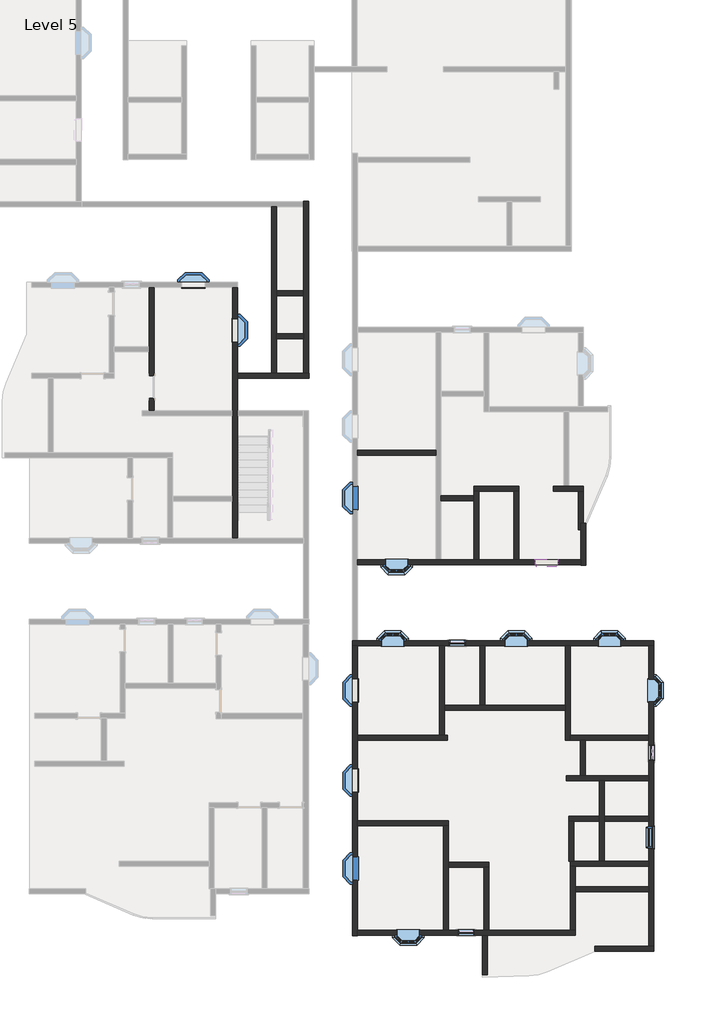
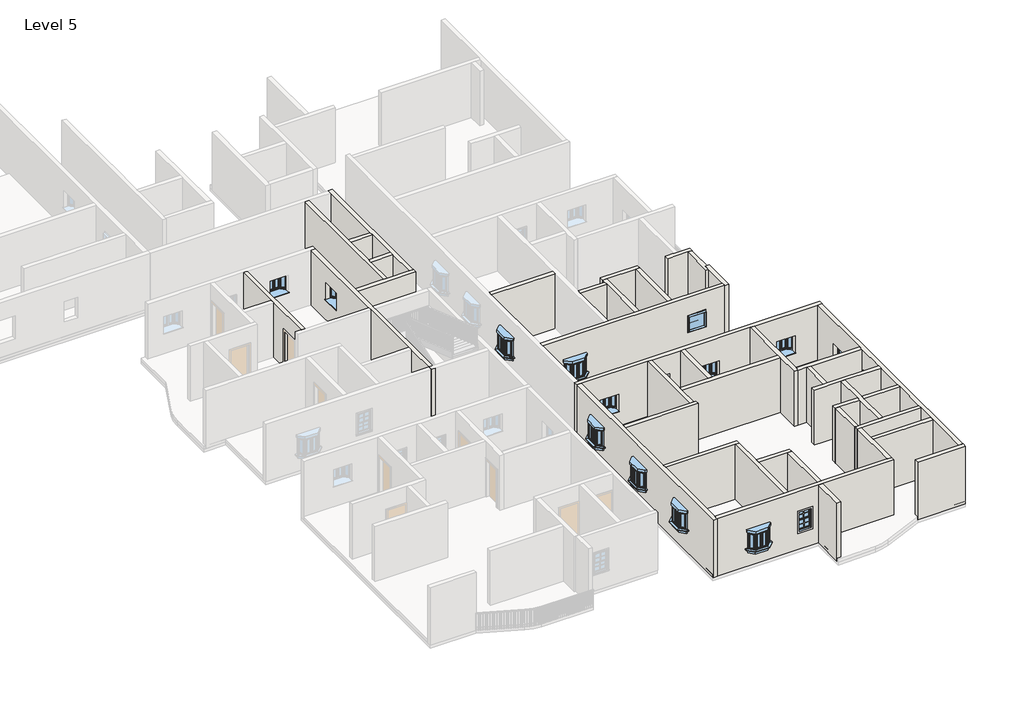
# One storey, part 2 of 14: 40 walls, 17 windows.
"""IFC4 building model written with IfcOpenShell, lengths in millimetres."""

from ifc_helpers import new_model, si_unit, frame, origin, place, context, project, spatial, polyline, outline, extrude, faceted_brep, transform, mapped, element, save
from components import window_910x910mm_67ef725a, window_8debb0fa, windows_sgl_w_glazing_bars_910x910mm_256712d0

model = new_model("IFC4")

# Units and contexts
model_context = context("Model", 3, world=origin())
ifc_project = project(units=[si_unit("LENGTHUNIT", "METRE", prefix="MILLI")], contexts=[model_context])

# Site, building, storey
site = spatial("IfcSite", under=ifc_project)
building = spatial("IfcBuilding", under=site)
storey = spatial("IfcBuildingStorey", under=building, Name="Level 5", Elevation=12192.0)

# Walls
placement = place(None, origin())
element("IfcWall", 1, ObjectType="4.5\" p", at=placement, inside=storey, context=model_context, shape_type="SweptSolid", body=[
    extrude(outline(polyline([(6070.4380523, -28382.7374148), (6070.4380523, -26796.6042694), (6273.6380523, -26796.6042694), (6273.6380523, -28382.7374148), (6070.4380523, -28382.7374148)])), frame((0.0, 0.0, 12192.0), z_axis=(0.0, 0.0, 1.0), x_axis=(1.0, 0.0, 0.0)), (0.0, 0.0, 1.0), 3048.0),
])
element("IfcWall", 2, ObjectType="4.5\" p", at=placement, inside=storey, context=model_context, shape_type="Brep", body=[
    faceted_brep([(10639.6896214, -27431.6042694, 12192.0), (13030.0380523, -27431.6042694, 12192.0), (13030.0380523, -27431.6042694, 15240.0), (10639.6896214, -27431.6042694, 15240.0), (10639.6896214, -27228.4042694, 12192.0), (10639.6896214, -27228.4042694, 15240.0), (12814.1380523, -27228.4042694, 15240.0), (13017.3380523, -27228.4042694, 15240.0), (13030.0380523, -27228.4042694, 15240.0), (13030.0380523, -27228.4042694, 12192.0), (13017.3380523, -27228.4042694, 12192.0), (12814.1380523, -27228.4042694, 12192.0)], [[[0, 1, 2, 3]], [[4, 5, 6, 7, 8, 9, 10, 11]], [[1, 0, 4, 11, 10, 9]], [[2, 1, 9, 8]], [[3, 2, 8, 7, 6, 5]], [[0, 3, 5, 4]]]),
])
element("IfcWall", 3, ObjectType="4.5\" p", at=placement, inside=storey, context=model_context, shape_type="Brep", body=[
    faceted_brep([(1015.8380523, -18878.1542694, 12192.0), (4648.0380523, -18878.1542694, 12192.0), (4648.0380523, -18878.1542694, 15240.0), (1015.8380523, -18878.1542694, 15240.0), (1015.8380523, -18674.9542694, 12192.0), (1015.8380523, -18674.9542694, 15240.0), (4336.8880523, -18674.9542694, 15240.0), (4540.0880523, -18674.9542694, 15240.0), (4648.0380523, -18674.9542694, 15240.0), (4648.0380523, -18674.9542694, 12192.0), (4540.0880523, -18674.9542694, 12192.0), (4336.8880523, -18674.9542694, 12192.0)], [[[0, 1, 2, 3]], [[4, 5, 6, 7, 8, 9, 10, 11]], [[1, 0, 4, 11, 10, 9]], [[2, 1, 9, 8]], [[3, 2, 8, 7, 6, 5]], [[0, 3, 5, 4]]]),
])
element("IfcWall", 4, ObjectType="4.5\" p", at=placement, inside=storey, context=model_context, shape_type="Brep", body=[
    faceted_brep([(4336.8880523, -15049.1042694, 12192.0), (4336.8880523, -18674.9542694, 12192.0), (4336.8880523, -18674.9542694, 15240.0), (4336.8880523, -15049.1042694, 15240.0), (4540.0880523, -15049.1042694, 12192.0), (4540.0880523, -15049.1042694, 15240.0), (4540.0880523, -17455.7542694, 15240.0), (4540.0880523, -17658.9542694, 15240.0), (4540.0880523, -18674.9542694, 15240.0), (4540.0880523, -18674.9542694, 12192.0), (4540.0880523, -17658.9542694, 12192.0), (4540.0880523, -17455.7542694, 12192.0)], [[[0, 1, 2, 3]], [[4, 5, 6, 7, 8, 9, 10, 11]], [[1, 0, 4, 11, 10, 9]], [[3, 2, 8, 7, 6, 5]], [[0, 3, 5, 4]], [[2, 1, 9, 8]]]),
])
element("IfcWall", 5, ObjectType="4.5\" p", at=placement, inside=storey, context=model_context, shape_type="Brep", body=[
    faceted_brep([(4540.0880523, -17658.9542694, 12192.0), (9442.2880523, -17658.9542694, 12192.0), (9442.2880523, -17658.9542694, 15240.0), (4540.0880523, -17658.9542694, 15240.0), (4540.0880523, -17455.7542694, 12192.0), (4540.0880523, -17455.7542694, 15240.0), (5975.1880523, -17455.7542694, 15240.0), (6178.3880523, -17455.7542694, 15240.0), (9442.2880523, -17455.7542694, 15240.0), (9442.2880523, -17455.7542694, 12192.0), (6178.3880523, -17455.7542694, 12192.0), (5975.1880523, -17455.7542694, 12192.0)], [[[0, 1, 2, 3]], [[4, 5, 6, 7, 8, 9, 10, 11]], [[1, 0, 4, 11, 10, 9]], [[3, 2, 8, 7, 6, 5]], [[0, 3, 5, 4]], [[2, 1, 9, 8]]]),
])
element("IfcWall", 6, ObjectType="4.5\" p", at=placement, inside=storey, context=model_context, shape_type="SweptSolid", body=[
    extrude(outline(polyline([(5975.1880523, -17455.7542694), (5975.1880523, -15049.1042694), (6178.3880523, -15049.1042694), (6178.3880523, -17455.7542694), (5975.1880523, -17455.7542694)])), frame((0.0, 0.0, 12192.0), z_axis=(0.0, 0.0, 1.0), x_axis=(1.0, 0.0, 0.0)), (0.0, 0.0, 1.0), 3048.0),
])
element("IfcWall", 7, ObjectType="4.5\" p", at=placement, inside=storey, context=model_context, shape_type="Brep", body=[
    faceted_brep([(9442.2880523, -15049.1042694, 12192.0), (9442.2880523, -17455.7542694, 12192.0), (9442.2880523, -17658.9542694, 12192.0), (9442.2880523, -18871.8042694, 12192.0), (9442.2880523, -18871.8042694, 15240.0), (9442.2880523, -17658.9542694, 15240.0), (9442.2880523, -17455.7542694, 15240.0), (9442.2880523, -15049.1042694, 15240.0), (9645.4880523, -15049.1042694, 12192.0), (9645.4880523, -15049.1042694, 15240.0), (9645.4880523, -18668.6042694, 15240.0), (9645.4880523, -18871.8042694, 15240.0), (9645.4880523, -18871.8042694, 12192.0), (9645.4880523, -18668.6042694, 12192.0)], [[[0, 1, 2, 3, 4, 5, 6, 7]], [[8, 9, 10, 11, 12, 13]], [[3, 2, 1, 0, 8, 13, 12]], [[7, 6, 5, 4, 11, 10, 9]], [[0, 7, 9, 8]], [[4, 3, 12, 11]]]),
])
element("IfcWall", 8, ObjectType="4.5\" p", at=placement, inside=storey, context=model_context, shape_type="Brep", body=[
    faceted_brep([(1015.8380523, -22345.2542694, 12192.0), (4489.2880523, -22345.2542694, 12192.0), (4692.4880523, -22345.2542694, 12192.0), (4692.4880523, -22345.2542694, 15240.0), (4489.2880523, -22345.2542694, 15240.0), (1015.8380523, -22345.2542694, 15240.0), (1015.8380523, -22142.0542694, 12192.0), (1015.8380523, -22142.0542694, 15240.0), (4692.4880523, -22142.0542694, 15240.0), (4692.4880523, -22142.0542694, 12192.0)], [[[0, 1, 2, 3, 4, 5]], [[6, 7, 8, 9]], [[2, 1, 0, 6, 9]], [[5, 4, 3, 8, 7]], [[0, 5, 7, 6]], [[3, 2, 9, 8]]]),
])
element("IfcWall", 9, ObjectType="4.5\" p", at=placement, inside=storey, context=model_context, shape_type="Brep", body=[
    faceted_brep([(4489.2880523, -22345.2542694, 12192.0), (4489.2880523, -26580.7042694, 12192.0), (4489.2880523, -26580.7042694, 15240.0), (4489.2880523, -22345.2542694, 15240.0), (4692.4880523, -22345.2542694, 12192.0), (4692.4880523, -22345.2542694, 15240.0), (4692.4880523, -23818.4542694, 15240.0), (4692.4880523, -24021.6542694, 15240.0), (4692.4880523, -26580.7042694, 15240.0), (4692.4880523, -26580.7042694, 12192.0), (4692.4880523, -24021.6542694, 12192.0), (4692.4880523, -23818.4542694, 12192.0)], [[[0, 1, 2, 3]], [[4, 5, 6, 7, 8, 9, 10, 11]], [[1, 0, 4, 11, 10, 9]], [[3, 2, 8, 7, 6, 5]], [[0, 3, 5, 4]], [[2, 1, 9, 8]]]),
])
element("IfcWall", 10, ObjectType="4.5\" p", at=placement, inside=storey, context=model_context, shape_type="Brep", body=[
    faceted_brep([(4692.4880523, -24021.6542694, 12192.0), (6127.5880523, -24021.6542694, 12192.0), (6330.7880523, -24021.6542694, 12192.0), (6330.7880523, -24021.6542694, 15240.0), (6127.5880523, -24021.6542694, 15240.0), (4692.4880523, -24021.6542694, 15240.0), (4692.4880523, -23818.4542694, 12192.0), (4692.4880523, -23818.4542694, 15240.0), (6330.7880523, -23818.4542694, 15240.0), (6330.7880523, -23818.4542694, 12192.0)], [[[0, 1, 2, 3, 4, 5]], [[6, 7, 8, 9]], [[2, 1, 0, 6, 9]], [[5, 4, 3, 8, 7]], [[0, 5, 7, 6]], [[3, 2, 9, 8]]]),
])
element("IfcWall", 11, ObjectType="4.5\" p", at=placement, inside=storey, context=model_context, shape_type="SweptSolid", body=[
    extrude(outline(polyline([(6127.5880523, -26580.7042694), (6127.5880523, -24021.6542694), (6330.7880523, -24021.6542694), (6330.7880523, -26580.7042694), (6127.5880523, -26580.7042694)])), frame((0.0, 0.0, 12192.0), z_axis=(0.0, 0.0, 1.0), x_axis=(1.0, 0.0, 0.0)), (0.0, 0.0, 1.0), 3048.0),
])
element("IfcWall", 12, ObjectType="4.5\" p", at=placement, inside=storey, context=model_context, shape_type="Brep", body=[
    faceted_brep([(9645.4880523, -18871.8042694, 12192.0), (10051.8880523, -18871.8042694, 12192.0), (10255.0880523, -18871.8042694, 12192.0), (12814.1380523, -18871.8042694, 12192.0), (12814.1380523, -18871.8042694, 15240.0), (10255.0880523, -18871.8042694, 15240.0), (10051.8880523, -18871.8042694, 15240.0), (9645.4880523, -18871.8042694, 15240.0), (9645.4880523, -18668.6042694, 12192.0), (9645.4880523, -18668.6042694, 15240.0), (12814.1380523, -18668.6042694, 15240.0), (12814.1380523, -18668.6042694, 12192.0)], [[[0, 1, 2, 3, 4, 5, 6, 7]], [[8, 9, 10, 11]], [[3, 2, 1, 0, 8, 11]], [[7, 6, 5, 4, 10, 9]], [[0, 7, 9, 8]], [[4, 3, 11, 10]]]),
])
element("IfcWall", 13, ObjectType="4.5\" p", at=placement, inside=storey, context=model_context, shape_type="SweptSolid", body=[
    extrude(outline(polyline([(10051.8880523, -20313.2542694), (10051.8880523, -18871.8042694), (10255.0880523, -18871.8042694), (10255.0880523, -20313.2542694), (10051.8880523, -20313.2542694)])), frame((0.0, 0.0, 12192.0), z_axis=(0.0, 0.0, 1.0), x_axis=(1.0, 0.0, 0.0)), (0.0, 0.0, 1.0), 3048.0),
])
element("IfcWall", 14, ObjectType="4.5\" p", at=placement, inside=storey, context=model_context, shape_type="Brep", body=[
    faceted_brep([(12814.1380523, -20313.2542694, 12192.0), (10255.0880523, -20313.2542694, 12192.0), (10051.8880523, -20313.2542694, 12192.0), (9486.7380523, -20313.2542694, 12192.0), (9486.7380523, -20313.2542694, 15240.0), (10051.8880523, -20313.2542694, 15240.0), (10255.0880523, -20313.2542694, 15240.0), (12814.1380523, -20313.2542694, 15240.0), (12814.1380523, -20516.4542694, 12192.0), (12814.1380523, -20516.4542694, 15240.0), (11017.0880523, -20516.4542694, 15240.0), (10813.8880523, -20516.4542694, 15240.0), (9486.7380523, -20516.4542694, 15240.0), (9486.7380523, -20516.4542694, 12192.0), (10813.8880523, -20516.4542694, 12192.0), (11017.0880523, -20516.4542694, 12192.0)], [[[0, 1, 2, 3, 4, 5, 6, 7]], [[8, 9, 10, 11, 12, 13, 14, 15]], [[3, 2, 1, 0, 8, 15, 14, 13]], [[4, 3, 13, 12]], [[7, 6, 5, 4, 12, 11, 10, 9]], [[0, 7, 9, 8]]]),
])
element("IfcWall", 15, ObjectType="4.5\" p", at=placement, inside=storey, context=model_context, shape_type="Brep", body=[
    faceted_brep([(10813.8880523, -20516.4542694, 12192.0), (10813.8880523, -21951.5542694, 12192.0), (10813.8880523, -22154.7542694, 12192.0), (10813.8880523, -23779.5416506, 12192.0), (10813.8880523, -23779.5416506, 15240.0), (10813.8880523, -22154.7542694, 15240.0), (10813.8880523, -21951.5542694, 15240.0), (10813.8880523, -20516.4542694, 15240.0), (11017.0880523, -20516.4542694, 12192.0), (11017.0880523, -20516.4542694, 15240.0), (11017.0880523, -21951.5542694, 15240.0), (11017.0880523, -22154.7542694, 15240.0), (11017.0880523, -23779.5416506, 15240.0), (11017.0880523, -23779.5416506, 12192.0), (11017.0880523, -22154.7542694, 12192.0), (11017.0880523, -21951.5542694, 12192.0)], [[[0, 1, 2, 3, 4, 5, 6, 7]], [[8, 9, 10, 11, 12, 13, 14, 15]], [[3, 2, 1, 0, 8, 15, 14, 13]], [[7, 6, 5, 4, 12, 11, 10, 9]], [[0, 7, 9, 8]], [[4, 3, 13, 12]]]),
])
element("IfcWall", 16, ObjectType="4.5\" p", at=placement, inside=storey, context=model_context, shape_type="Brep", body=[
    faceted_brep([(12814.1380523, -23779.5416506, 12192.0), (11017.0880523, -23779.5416506, 12192.0), (10813.8880523, -23779.5416506, 12192.0), (9791.5380523, -23779.5416506, 12192.0), (9632.7880523, -23779.5416506, 12192.0), (9632.7880523, -23779.5416506, 15240.0), (9791.5380523, -23779.5416506, 15240.0), (10813.8880523, -23779.5416506, 15240.0), (11017.0880523, -23779.5416506, 15240.0), (12814.1380523, -23779.5416506, 15240.0), (12814.1380523, -23982.7416506, 12192.0), (12814.1380523, -23982.7416506, 15240.0), (9835.9880523, -23982.7416506, 15240.0), (9632.7880523, -23982.7416506, 15240.0), (9632.7880523, -23982.7416506, 12192.0), (9835.9880523, -23982.7416506, 12192.0)], [[[0, 1, 2, 3, 4, 5, 6, 7, 8, 9]], [[10, 11, 12, 13, 14, 15]], [[4, 3, 2, 1, 0, 10, 15, 14]], [[9, 8, 7, 6, 5, 13, 12, 11]], [[0, 9, 11, 10]], [[5, 4, 14, 13]]]),
])
element("IfcWall", 17, ObjectType="4.5\" p", at=placement, inside=storey, context=model_context, shape_type="Brep", body=[
    faceted_brep([(9632.7880523, -23982.7416506, 12192.0), (9632.7880523, -26580.7042694, 12192.0), (9632.7880523, -26580.7042694, 15240.0), (9632.7880523, -23982.7416506, 15240.0), (9835.9880523, -23982.7416506, 12192.0), (9835.9880523, -23982.7416506, 15240.0), (9835.9880523, -24805.3496998, 15240.0), (9835.9880523, -25008.5496998, 15240.0), (9835.9880523, -26580.7042694, 15240.0), (9835.9880523, -26580.7042694, 12192.0), (9835.9880523, -25008.5496998, 12192.0), (9835.9880523, -24805.3496998, 12192.0)], [[[0, 1, 2, 3]], [[4, 5, 6, 7, 8, 9, 10, 11]], [[1, 0, 4, 11, 10, 9]], [[3, 2, 8, 7, 6, 5]], [[2, 1, 9, 8]], [[0, 3, 5, 4]]]),
])
element("IfcWall", 18, ObjectType="4.5\" p", at=placement, inside=storey, context=model_context, shape_type="SweptSolid", body=[
    extrude(outline(polyline([(12814.1380523, -25008.5496998), (9835.9880523, -25008.5496998), (9835.9880523, -24805.3496998), (12814.1380523, -24805.3496998), (12814.1380523, -25008.5496998)])), frame((0.0, 0.0, 12192.0), z_axis=(0.0, 0.0, 1.0), x_axis=(1.0, 0.0, 0.0)), (0.0, 0.0, 1.0), 3048.0),
])
element("IfcWall", 19, ObjectType="4.5\" p", at=placement, inside=storey, context=model_context, shape_type="Brep", body=[
    faceted_brep([(-7432.737215, -5015.2916506, 14325.6), (-7432.737215, -5015.2916506, 12192.0), (-7432.737215, -5523.2916506, 12192.0), (-7432.737215, -5523.2916506, 15240.0), (-7432.737215, -3135.6916506, 15240.0), (-7432.737215, -2932.4916506, 15240.0), (-7432.737215, -525.8416506, 15240.0), (-7432.737215, -525.8416506, 12192.0), (-7432.737215, -2932.4916506, 12192.0), (-7432.737215, -3135.6916506, 12192.0), (-7432.737215, -4100.8916506, 12192.0), (-7432.737215, -4100.8916506, 14325.6), (-7229.537215, -5523.2916506, 12192.0), (-7229.537215, -5015.2916506, 12192.0), (-7229.537215, -5015.2916506, 14325.6), (-7229.537215, -4100.8916506, 14325.6), (-7229.537215, -4100.8916506, 12192.0), (-7229.537215, -525.8416506, 12192.0), (-7229.537215, -525.8416506, 15240.0), (-7229.537215, -5523.2916506, 15240.0)], [[[0, 1, 2, 3, 4, 5, 6, 7, 8, 9, 10, 11]], [[12, 13, 14, 15, 16, 17, 18, 19]], [[2, 1, 13, 12]], [[10, 9, 8, 7, 17, 16]], [[6, 5, 4, 3, 19, 18]], [[7, 6, 18, 17]], [[3, 2, 12, 19]], [[14, 13, 1, 0]], [[15, 14, 0, 11]], [[16, 15, 11, 10]]]),
])
element("IfcWall", 20, ObjectType="4.5\" p", at=placement, inside=storey, context=model_context, shape_type="Brep", body=[
    faceted_brep([(-3857.687215, -4202.4916506, 12192.0), (-961.4891351, -4202.4916506, 12192.0), (-961.4891351, -4202.4916506, 15240.0), (-3857.687215, -4202.4916506, 15240.0), (-3857.687215, -3999.2916506, 12192.0), (-3857.687215, -3999.2916506, 15240.0), (-2472.7891351, -3999.2916506, 15240.0), (-2269.5891351, -3999.2916506, 15240.0), (-1177.3891351, -3999.2916506, 15240.0), (-974.1891351, -3999.2916506, 15240.0), (-961.4891351, -3999.2916506, 15240.0), (-961.4891351, -3999.2916506, 12192.0), (-974.1891351, -3999.2916506, 12192.0), (-1177.3891351, -3999.2916506, 12192.0), (-2269.5891351, -3999.2916506, 12192.0), (-2472.7891351, -3999.2916506, 12192.0)], [[[0, 1, 2, 3]], [[4, 5, 6, 7, 8, 9, 10, 11, 12, 13, 14, 15]], [[1, 0, 4, 15, 14, 13, 12, 11]], [[2, 1, 11, 10]], [[3, 2, 10, 9, 8, 7, 6, 5]], [[0, 3, 5, 4]]]),
])
element("IfcWall", 21, ObjectType="4.5\" p", at=placement, inside=storey, context=model_context, shape_type="SweptSolid", body=[
    extrude(outline(polyline([(-1177.3891351, -868.7416506), (-2269.5891351, -868.7416506), (-2269.5891351, -665.5416506), (-1177.3891351, -665.5416506), (-1177.3891351, -868.7416506)])), frame((0.0, 0.0, 12192.0), z_axis=(0.0, 0.0, 1.0), x_axis=(1.0, 0.0, 0.0)), (0.0, 0.0, 1.0), 3048.0),
])
element("IfcWall", 22, ObjectType="4.5\" p", at=placement, inside=storey, context=model_context, shape_type="SweptSolid", body=[
    extrude(outline(polyline([(-1177.3891351, -2597.8466506), (-2269.5891351, -2597.8466506), (-2269.5891351, -2394.6466506), (-1177.3891351, -2394.6466506), (-1177.3891351, -2597.8466506)])), frame((0.0, 0.0, 12192.0), z_axis=(0.0, 0.0, 1.0), x_axis=(1.0, 0.0, 0.0)), (0.0, 0.0, 1.0), 3048.0),
])
element("IfcWall", 23, ObjectType="4.5\" p", at=placement, inside=storey, context=model_context, shape_type="SweptSolid", body=[
    extrude(outline(polyline([(5721.1880523, -9162.6542694), (4387.6880523, -9162.6542694), (4387.6880523, -8959.4542694), (5721.1880523, -8959.4542694), (5721.1880523, -9162.6542694)])), frame((0.0, 0.0, 12192.0), z_axis=(0.0, 0.0, 1.0), x_axis=(1.0, 0.0, 0.0)), (0.0, 0.0, 1.0), 3048.0),
])
element("IfcWall", 24, ObjectType="4.5\" p", at=placement, inside=storey, context=model_context, shape_type="Brep", body=[
    faceted_brep([(5721.1880523, -8781.6542694, 12192.0), (5924.3880523, -8781.6542694, 12192.0), (7359.4880523, -8781.6542694, 12192.0), (7562.6880523, -8781.6542694, 12192.0), (7562.6880523, -8781.6542694, 15240.0), (7359.4880523, -8781.6542694, 15240.0), (5924.3880523, -8781.6542694, 15240.0), (5721.1880523, -8781.6542694, 15240.0), (5721.1880523, -8578.4542694, 12192.0), (5721.1880523, -8578.4542694, 15240.0), (7562.6880523, -8578.4542694, 15240.0), (7562.6880523, -8578.4542694, 12192.0)], [[[0, 1, 2, 3, 4, 5, 6, 7]], [[8, 9, 10, 11]], [[3, 2, 1, 0, 8, 11]], [[7, 6, 5, 4, 10, 9]], [[0, 7, 9, 8]], [[4, 3, 11, 10]]]),
])
element("IfcWall", 25, ObjectType="4.5\" p", at=placement, inside=storey, context=model_context, shape_type="Brep", body=[
    faceted_brep([(5721.1880523, -8781.6542694, 12192.0), (5721.1880523, -8959.4542694, 12192.0), (5721.1880523, -9162.6542694, 12192.0), (5721.1880523, -11556.6042694, 12192.0), (5721.1880523, -11556.6042694, 15240.0), (5721.1880523, -9162.6542694, 15240.0), (5721.1880523, -8959.4542694, 15240.0), (5721.1880523, -8781.6542694, 15240.0), (5924.3880523, -8781.6542694, 12192.0), (5924.3880523, -8781.6542694, 15240.0), (5924.3880523, -11556.6042694, 15240.0), (5924.3880523, -11556.6042694, 12192.0)], [[[0, 1, 2, 3, 4, 5, 6, 7]], [[8, 9, 10, 11]], [[3, 2, 1, 0, 8, 11]], [[7, 6, 5, 4, 10, 9]], [[0, 7, 9, 8]], [[4, 3, 11, 10]]]),
])
element("IfcWall", 26, ObjectType="4.5\" p", at=placement, inside=storey, context=model_context, shape_type="SweptSolid", body=[
    extrude(outline(polyline([(7359.4880523, -11556.6042694), (7359.4880523, -8781.6542694), (7562.6880523, -8781.6542694), (7562.6880523, -11556.6042694), (7359.4880523, -11556.6042694)])), frame((0.0, 0.0, 12192.0), z_axis=(0.0, 0.0, 1.0), x_axis=(1.0, 0.0, 0.0)), (0.0, 0.0, 1.0), 3048.0),
])
element("IfcWall", 27, ObjectType="4.5\" p", at=placement, inside=storey, context=model_context, shape_type="SweptSolid", body=[
    extrude(outline(polyline([(4184.4880523, -7333.8542694), (1007.0108649, -7333.8542694), (1007.0108649, -7130.6542694), (4184.4880523, -7130.6542694), (4184.4880523, -7333.8542694)])), frame((0.0, 0.0, 12192.0), z_axis=(0.0, 0.0, 1.0), x_axis=(1.0, 0.0, 0.0)), (0.0, 0.0, 1.0), 3048.0),
])
element("IfcWall", 28, ObjectType="4.5\" p", at=placement, inside=storey, context=model_context, shape_type="Brep", body=[
    faceted_brep([(8953.3380523, -8781.6542694, 12192.0), (9956.6380523, -8781.6542694, 12192.0), (10159.8380523, -8781.6542694, 12192.0), (10172.5380523, -8781.6542694, 12192.0), (10172.5380523, -8781.6542694, 15240.0), (10159.8380523, -8781.6542694, 15240.0), (9956.6380523, -8781.6542694, 15240.0), (8953.3380523, -8781.6542694, 15240.0), (8953.3380523, -8578.4542694, 12192.0), (8953.3380523, -8578.4542694, 15240.0), (9371.2322031, -8578.4542694, 15240.0), (9574.4322031, -8578.4542694, 15240.0), (10172.5380523, -8578.4542694, 15240.0), (10172.5380523, -8578.4542694, 12192.0), (9574.4322031, -8578.4542694, 12192.0), (9371.2322031, -8578.4542694, 12192.0)], [[[0, 1, 2, 3, 4, 5, 6, 7]], [[8, 9, 10, 11, 12, 13, 14, 15]], [[3, 2, 1, 0, 8, 15, 14, 13]], [[4, 3, 13, 12]], [[7, 6, 5, 4, 12, 11, 10, 9]], [[0, 7, 9, 8]]]),
])
element("IfcWall", 29, ObjectType="4.5\" p", at=placement, inside=storey, context=model_context, shape_type="SweptSolid", body=[
    extrude(outline(polyline([(9956.6380523, -10352.8912671), (9956.6380523, -8781.6542694), (10159.8380523, -8781.6542694), (10159.8380523, -10352.8912671), (9956.6380523, -10352.8912671)])), frame((0.0, 0.0, 12192.0), z_axis=(0.0, 0.0, 1.0), x_axis=(1.0, 0.0, 0.0)), (0.0, 0.0, 1.0), 3048.0),
])
element("IfcWall", 30, ObjectType="4.5\" p", at=placement, inside=storey, context=model_context, shape_type="Brep", body=[
    faceted_brep([(12814.1380523, -21951.5542694, 15240.0), (12814.1380523, -21951.5542694, 12192.0), (11017.0880523, -21951.5542694, 12192.0), (11017.0880523, -21951.5542694, 15240.0), (12814.1380523, -22154.7542694, 12192.0), (12814.1380523, -22154.7542694, 15240.0), (11017.0880523, -22154.7542694, 15240.0), (11017.0880523, -22154.7542694, 12192.0)], [[[0, 1, 2, 3]], [[4, 5, 6, 7]], [[1, 4, 7, 2]], [[5, 0, 3, 6]], [[1, 0, 5, 4]], [[3, 2, 7, 6]]]),
    faceted_brep([(9588.3380523, -21951.5542694, 12192.0), (9588.3380523, -21951.5542694, 15240.0), (10813.8880523, -21951.5542694, 15240.0), (10813.8880523, -21951.5542694, 12192.0), (9588.3380523, -22154.7542694, 15240.0), (9588.3380523, -22154.7542694, 12192.0), (9791.5380523, -22154.7542694, 12192.0), (10813.8880523, -22154.7542694, 12192.0), (10813.8880523, -22154.7542694, 15240.0), (9791.5380523, -22154.7542694, 15240.0)], [[[0, 1, 2, 3]], [[4, 5, 6, 7, 8, 9]], [[5, 0, 3, 7, 6]], [[1, 4, 9, 8, 2]], [[3, 2, 8, 7]], [[1, 0, 5, 4]]]),
])
element("IfcWall", 31, ObjectType="4.5\" p", at=placement, inside=storey, context=model_context, shape_type="Brep", body=[
    faceted_brep([(9588.3380523, -22154.7542694, 12192.0), (9588.3380523, -23779.5416506, 12192.0), (9588.3380523, -23779.5416506, 15240.0), (9588.3380523, -22154.7542694, 15240.0), (9791.5380523, -22154.7542694, 12192.0), (9791.5380523, -22154.7542694, 15240.0), (9791.5380523, -23779.5416506, 15240.0), (9791.5380523, -23779.5416506, 12192.0), (9632.7880523, -23779.5416506, 12192.0), (9632.7880523, -23779.5416506, 15240.0)], [[[0, 1, 2, 3]], [[4, 5, 6, 7]], [[1, 0, 4, 7, 8]], [[3, 2, 9, 6, 5]], [[2, 1, 8, 7, 6, 9]], [[0, 3, 5, 4]]]),
])
element("IfcWall", 32, ObjectType="9\"", at=placement, inside=storey, context=model_context, shape_type="Brep", body=[
    faceted_brep([(799.9380523, -15049.1042694, 12192.0), (812.6380523, -15049.1042694, 12192.0), (1015.8380523, -15049.1042694, 12192.0), (4336.8880523, -15049.1042694, 12192.0), (4540.0880523, -15049.1042694, 12192.0), (5975.1880523, -15049.1042694, 12192.0), (6178.3880523, -15049.1042694, 12192.0), (9442.2880523, -15049.1042694, 12192.0), (9645.4880523, -15049.1042694, 12192.0), (12814.1380523, -15049.1042694, 12192.0), (13017.3380523, -15049.1042694, 12192.0), (13030.0380523, -15049.1042694, 12192.0), (13030.0380523, -15049.1042694, 15240.0), (13017.3380523, -15049.1042694, 15240.0), (12814.1380523, -15049.1042694, 15240.0), (9645.4880523, -15049.1042694, 15240.0), (9442.2880523, -15049.1042694, 15240.0), (6178.3880523, -15049.1042694, 15240.0), (5975.1880523, -15049.1042694, 15240.0), (4540.0880523, -15049.1042694, 15240.0), (4336.8880523, -15049.1042694, 15240.0), (1015.8380523, -15049.1042694, 15240.0), (812.6380523, -15049.1042694, 15240.0), (799.9380523, -15049.1042694, 15240.0), (1983.2380523, -15049.1042694, 14016.4), (2893.2380523, -15049.1042694, 14016.4), (2893.2380523, -15049.1042694, 13106.4), (1983.2380523, -15049.1042694, 13106.4), (10774.8130523, -15049.1042694, 14016.4), (11684.8130523, -15049.1042694, 14016.4), (11684.8130523, -15049.1042694, 13106.4), (10774.8130523, -15049.1042694, 13106.4), (6993.3880523, -15049.1042694, 14016.4), (7903.3880523, -15049.1042694, 14016.4), (7903.3880523, -15049.1042694, 13106.4), (6993.3880523, -15049.1042694, 13106.4), (4717.8880523, -15049.1042694, 14173.2), (5378.2880523, -15049.1042694, 14173.2), (5378.2880523, -15049.1042694, 13106.4), (4717.8880523, -15049.1042694, 13106.4), (799.9380523, -14845.9042694, 12192.0), (799.9380523, -14845.9042694, 15240.0), (803.8108649, -14845.9042694, 15240.0), (1007.0108649, -14845.9042694, 15240.0), (13030.0380523, -14845.9042694, 15240.0), (13030.0380523, -14845.9042694, 12192.0), (1007.0108649, -14845.9042694, 12192.0), (803.8108649, -14845.9042694, 12192.0), (1983.2380523, -14845.9042694, 14016.4), (1983.2380523, -14845.9042694, 13106.4), (2893.2380523, -14845.9042694, 13106.4), (2893.2380523, -14845.9042694, 14016.4), (10774.8130523, -14845.9042694, 14016.4), (10774.8130523, -14845.9042694, 13106.4), (11684.8130523, -14845.9042694, 13106.4), (11684.8130523, -14845.9042694, 14016.4), (6993.3880523, -14845.9042694, 14016.4), (6993.3880523, -14845.9042694, 13106.4), (7903.3880523, -14845.9042694, 13106.4), (7903.3880523, -14845.9042694, 14016.4), (4717.8880523, -14845.9042694, 14173.2), (4717.8880523, -14845.9042694, 13106.4), (5378.2880523, -14845.9042694, 13106.4), (5378.2880523, -14845.9042694, 14173.2)], [[[0, 1, 2, 3, 4, 5, 6, 7, 8, 9, 10, 11, 12, 13, 14, 15, 16, 17, 18, 19, 20, 21, 22, 23], [24, 25, 26, 27], [28, 29, 30, 31], [32, 33, 34, 35], [36, 37, 38, 39]], [[40, 41, 42, 43, 44, 45, 46, 47], [48, 49, 50, 51], [52, 53, 54, 55], [56, 57, 58, 59], [60, 61, 62, 63]], [[11, 10, 9, 8, 7, 6, 5, 4, 3, 2, 1, 0, 40, 47, 46, 45]], [[12, 11, 45, 44]], [[23, 22, 21, 20, 19, 18, 17, 16, 15, 14, 13, 12, 44, 43, 42, 41]], [[0, 23, 41, 40]], [[49, 48, 24, 27]], [[50, 49, 27, 26]], [[51, 50, 26, 25]], [[48, 51, 25, 24]], [[53, 52, 28, 31]], [[54, 53, 31, 30]], [[55, 54, 30, 29]], [[52, 55, 29, 28]], [[57, 56, 32, 35]], [[58, 57, 35, 34]], [[59, 58, 34, 33]], [[56, 59, 33, 32]], [[61, 60, 36, 39]], [[62, 61, 39, 38]], [[63, 62, 38, 37]], [[60, 63, 37, 36]]]),
])
element("IfcWall", 33, ObjectType="9\"", at=placement, inside=storey, context=model_context, shape_type="Brep", body=[
    faceted_brep([(12814.1380523, -15049.1042694, 12192.0), (12814.1380523, -18668.6042694, 12192.0), (12814.1380523, -18871.8042694, 12192.0), (12814.1380523, -20313.2542694, 12192.0), (12814.1380523, -20516.4542694, 12192.0), (12814.1380523, -21951.5542694, 12192.0), (12814.1380523, -22154.7542694, 12192.0), (12814.1380523, -23779.5416506, 12192.0), (12814.1380523, -23982.7416506, 12192.0), (12814.1380523, -24805.3496998, 12192.0), (12814.1380523, -25008.5496998, 12192.0), (12814.1380523, -27228.4042694, 12192.0), (12814.1380523, -27228.4042694, 15240.0), (12814.1380523, -25008.5496998, 15240.0), (12814.1380523, -24805.3496998, 15240.0), (12814.1380523, -23982.7416506, 15240.0), (12814.1380523, -23779.5416506, 15240.0), (12814.1380523, -22154.7542694, 15240.0), (12814.1380523, -21951.5542694, 15240.0), (12814.1380523, -20516.4542694, 15240.0), (12814.1380523, -20313.2542694, 15240.0), (12814.1380523, -18871.8042694, 15240.0), (12814.1380523, -18668.6042694, 15240.0), (12814.1380523, -15049.1042694, 15240.0), (12814.1380523, -16403.8542694, 14016.4), (12814.1380523, -17313.8542694, 14016.4), (12814.1380523, -17313.8542694, 13106.4), (12814.1380523, -16403.8542694, 13106.4), (12814.1380523, -23270.1542694, 14016.4), (12814.1380523, -23270.1542694, 13106.4), (12814.1380523, -22360.1542694, 13106.4), (12814.1380523, -22360.1542694, 14016.4), (12814.1380523, -19049.6042694, 14173.2), (12814.1380523, -19710.0042694, 14173.2), (12814.1380523, -19710.0042694, 13106.4), (12814.1380523, -19049.6042694, 13106.4), (13017.3380523, -15049.1042694, 12192.0), (13017.3380523, -15049.1042694, 15240.0), (13017.3380523, -27228.4042694, 15240.0), (13017.3380523, -27228.4042694, 12192.0), (13017.3380523, -16403.8542694, 14016.4), (13017.3380523, -16403.8542694, 13106.4), (13017.3380523, -17313.8542694, 13106.4), (13017.3380523, -17313.8542694, 14016.4), (13017.3380523, -23270.1542694, 14016.4), (13017.3380523, -22360.1542694, 14016.4), (13017.3380523, -22360.1542694, 13106.4), (13017.3380523, -23270.1542694, 13106.4), (13017.3380523, -19049.6042694, 14173.2), (13017.3380523, -19049.6042694, 13106.4), (13017.3380523, -19710.0042694, 13106.4), (13017.3380523, -19710.0042694, 14173.2)], [[[0, 1, 2, 3, 4, 5, 6, 7, 8, 9, 10, 11, 12, 13, 14, 15, 16, 17, 18, 19, 20, 21, 22, 23], [24, 25, 26, 27], [28, 29, 30, 31], [32, 33, 34, 35]], [[36, 37, 38, 39], [40, 41, 42, 43], [44, 45, 46, 47], [48, 49, 50, 51]], [[11, 10, 9, 8, 7, 6, 5, 4, 3, 2, 1, 0, 36, 39]], [[23, 22, 21, 20, 19, 18, 17, 16, 15, 14, 13, 12, 38, 37]], [[0, 23, 37, 36]], [[12, 11, 39, 38]], [[41, 40, 24, 27]], [[42, 41, 27, 26]], [[43, 42, 26, 25]], [[40, 43, 25, 24]], [[29, 28, 44, 47]], [[30, 29, 47, 46]], [[31, 30, 46, 45]], [[28, 31, 45, 44]], [[49, 48, 32, 35]], [[50, 49, 35, 34]], [[51, 50, 34, 33]], [[48, 51, 33, 32]]]),
])
element("IfcWall", 34, ObjectType="9\"", at=placement, inside=storey, context=model_context, shape_type="Brep", body=[
    faceted_brep([(812.6380523, -15049.1042694, 12192.0), (812.6380523, -26796.6042694, 12192.0), (812.6380523, -26796.6042694, 15240.0), (812.6380523, -15049.1042694, 15240.0), (812.6380523, -24527.4542694, 14302.0), (812.6380523, -24527.4542694, 13392.0), (812.6380523, -23617.4542694, 13392.0), (812.6380523, -23617.4542694, 14302.0), (812.6380523, -20965.1042694, 14302.0), (812.6380523, -20965.1042694, 13392.0), (812.6380523, -20055.1042694, 13392.0), (812.6380523, -20055.1042694, 14302.0), (812.6380523, -17317.0292694, 14302.0), (812.6380523, -17317.0292694, 13392.0), (812.6380523, -16407.0292694, 13392.0), (812.6380523, -16407.0292694, 14302.0), (1015.8380523, -15049.1042694, 12192.0), (1015.8380523, -15049.1042694, 15240.0), (1015.8380523, -18674.9542694, 15240.0), (1015.8380523, -18878.1542694, 15240.0), (1015.8380523, -22142.0542694, 15240.0), (1015.8380523, -22345.2542694, 15240.0), (1015.8380523, -26580.7042694, 15240.0), (1015.8380523, -26783.9042694, 15240.0), (1015.8380523, -26796.6042694, 15240.0), (1015.8380523, -26796.6042694, 12192.0), (1015.8380523, -26783.9042694, 12192.0), (1015.8380523, -26580.7042694, 12192.0), (1015.8380523, -22345.2542694, 12192.0), (1015.8380523, -22142.0542694, 12192.0), (1015.8380523, -18878.1542694, 12192.0), (1015.8380523, -18674.9542694, 12192.0), (1015.8380523, -24527.4542694, 14302.0), (1015.8380523, -23617.4542694, 14302.0), (1015.8380523, -23617.4542694, 13392.0), (1015.8380523, -24527.4542694, 13392.0), (1015.8380523, -20965.1042694, 14302.0), (1015.8380523, -20055.1042694, 14302.0), (1015.8380523, -20055.1042694, 13392.0), (1015.8380523, -20965.1042694, 13392.0), (1015.8380523, -17317.0292694, 14302.0), (1015.8380523, -16407.0292694, 14302.0), (1015.8380523, -16407.0292694, 13392.0), (1015.8380523, -17317.0292694, 13392.0)], [[[0, 1, 2, 3], [4, 5, 6, 7], [8, 9, 10, 11], [12, 13, 14, 15]], [[16, 17, 18, 19, 20, 21, 22, 23, 24, 25, 26, 27, 28, 29, 30, 31], [32, 33, 34, 35], [36, 37, 38, 39], [40, 41, 42, 43]], [[1, 0, 16, 31, 30, 29, 28, 27, 26, 25]], [[2, 1, 25, 24]], [[3, 2, 24, 23, 22, 21, 20, 19, 18, 17]], [[0, 3, 17, 16]], [[5, 4, 32, 35]], [[6, 5, 35, 34]], [[7, 6, 34, 33]], [[4, 7, 33, 32]], [[9, 8, 36, 39]], [[10, 9, 39, 38]], [[11, 10, 38, 37]], [[8, 11, 37, 36]], [[13, 12, 40, 43]], [[14, 13, 43, 42]], [[15, 14, 42, 41]], [[12, 15, 41, 40]]]),
])
element("IfcWall", 35, ObjectType="9\"", at=placement, inside=storey, context=model_context, shape_type="Brep", body=[
    faceted_brep([(1015.8380523, -26783.9042694, 12192.0), (9835.9880523, -26783.9042694, 12192.0), (9835.9880523, -26783.9042694, 15240.0), (1015.8380523, -26783.9042694, 15240.0), (3521.8880523, -26783.9042694, 14016.4), (3521.8880523, -26783.9042694, 13106.4), (2611.8880523, -26783.9042694, 13106.4), (2611.8880523, -26783.9042694, 14016.4), (5079.8380523, -26783.9042694, 14173.2), (5740.2380523, -26783.9042694, 14173.2), (5740.2380523, -26783.9042694, 13106.4), (5079.8380523, -26783.9042694, 13106.4), (1015.8380523, -26580.7042694, 12192.0), (1015.8380523, -26580.7042694, 15240.0), (4489.2880523, -26580.7042694, 15240.0), (4692.4880523, -26580.7042694, 15240.0), (6127.5880523, -26580.7042694, 15240.0), (6330.7880523, -26580.7042694, 15240.0), (9632.7880523, -26580.7042694, 15240.0), (9835.9880523, -26580.7042694, 15240.0), (9835.9880523, -26580.7042694, 12192.0), (9632.7880523, -26580.7042694, 12192.0), (6330.7880523, -26580.7042694, 12192.0), (6127.5880523, -26580.7042694, 12192.0), (4692.4880523, -26580.7042694, 12192.0), (4489.2880523, -26580.7042694, 12192.0), (3521.8880523, -26580.7042694, 14016.4), (2611.8880523, -26580.7042694, 14016.4), (2611.8880523, -26580.7042694, 13106.4), (3521.8880523, -26580.7042694, 13106.4), (5079.8380523, -26580.7042694, 14173.2), (5079.8380523, -26580.7042694, 13106.4), (5740.2380523, -26580.7042694, 13106.4), (5740.2380523, -26580.7042694, 14173.2)], [[[0, 1, 2, 3], [4, 5, 6, 7], [8, 9, 10, 11]], [[12, 13, 14, 15, 16, 17, 18, 19, 20, 21, 22, 23, 24, 25], [26, 27, 28, 29], [30, 31, 32, 33]], [[1, 0, 12, 25, 24, 23, 22, 21, 20]], [[3, 2, 19, 18, 17, 16, 15, 14, 13]], [[0, 3, 13, 12]], [[2, 1, 20, 19]], [[5, 4, 26, 29]], [[6, 5, 29, 28]], [[7, 6, 28, 27]], [[4, 7, 27, 26]], [[31, 30, 8, 11]], [[32, 31, 11, 10]], [[33, 32, 10, 9]], [[30, 33, 9, 8]]]),
])
element("IfcWall", 36, ObjectType="9\" w", at=placement, inside=storey, context=model_context, shape_type="Brep", body=[
    faceted_brep([(-4060.887215, -525.8416506, 12192.0), (-4060.887215, -5523.2916506, 12192.0), (-4060.887215, -5726.4916506, 12192.0), (-4060.887215, -8990.3916506, 12192.0), (-4060.887215, -9193.5916506, 12192.0), (-4060.887215, -10901.7416506, 12192.0), (-4060.887215, -10901.7416506, 15240.0), (-4060.887215, -9193.5916506, 15240.0), (-4060.887215, -8990.3916506, 15240.0), (-4060.887215, -5726.4916506, 15240.0), (-4060.887215, -5523.2916506, 15240.0), (-4060.887215, -525.8416506, 15240.0), (-4060.887215, -1807.5666506, 14302.0), (-4060.887215, -2717.5666506, 14302.0), (-4060.887215, -2717.5666506, 13392.0), (-4060.887215, -1807.5666506, 13392.0), (-3857.687215, -525.8416506, 12192.0), (-3857.687215, -525.8416506, 15240.0), (-3857.687215, -3999.2916506, 15240.0), (-3857.687215, -4202.4916506, 15240.0), (-3857.687215, -5523.2916506, 15240.0), (-3857.687215, -5726.4916506, 15240.0), (-3857.687215, -10901.7416506, 15240.0), (-3857.687215, -10901.7416506, 12192.0), (-3857.687215, -5726.4916506, 12192.0), (-3857.687215, -5523.2916506, 12192.0), (-3857.687215, -4202.4916506, 12192.0), (-3857.687215, -3999.2916506, 12192.0), (-3857.687215, -1807.5666506, 14302.0), (-3857.687215, -1807.5666506, 13392.0), (-3857.687215, -2717.5666506, 13392.0), (-3857.687215, -2717.5666506, 14302.0)], [[[0, 1, 2, 3, 4, 5, 6, 7, 8, 9, 10, 11], [12, 13, 14, 15]], [[16, 17, 18, 19, 20, 21, 22, 23, 24, 25, 26, 27], [28, 29, 30, 31]], [[5, 4, 3, 2, 1, 0, 16, 27, 26, 25, 24, 23]], [[6, 5, 23, 22]], [[11, 10, 9, 8, 7, 6, 22, 21, 20, 19, 18, 17]], [[0, 11, 17, 16]], [[29, 28, 12, 15]], [[30, 29, 15, 14]], [[31, 30, 14, 13]], [[28, 31, 13, 12]]]),
])
element("IfcWall", 37, ObjectType="9\" w", at=placement, inside=storey, context=model_context, shape_type="Brep", body=[
    faceted_brep([(-2269.5891351, -3999.2916506, 12192.0), (-2269.5891351, -2597.8466506, 12192.0), (-2269.5891351, -2394.6466506, 12192.0), (-2269.5891351, -868.7416506, 12192.0), (-2269.5891351, -665.5416506, 12192.0), (-2269.5891351, 2750.7583494, 12192.0), (-2269.5891351, 2750.7583494, 15240.0), (-2269.5891351, -665.5416506, 15240.0), (-2269.5891351, -868.7416506, 15240.0), (-2269.5891351, -2394.6466506, 15240.0), (-2269.5891351, -2597.8466506, 15240.0), (-2269.5891351, -3999.2916506, 15240.0), (-2472.7891351, -3999.2916506, 12192.0), (-2472.7891351, -3999.2916506, 15240.0), (-2472.7891351, 2750.7583494, 15240.0), (-2472.7891351, 2750.7583494, 12192.0)], [[[0, 1, 2, 3, 4, 5, 6, 7, 8, 9, 10, 11]], [[12, 13, 14, 15]], [[5, 4, 3, 2, 1, 0, 12, 15]], [[11, 10, 9, 8, 7, 6, 14, 13]], [[0, 11, 13, 12]], [[6, 5, 15, 14]]]),
])
element("IfcWall", 38, ObjectType="9\" w", at=placement, inside=storey, context=model_context, shape_type="Brep", body=[
    faceted_brep([(-974.1891351, -3999.2916506, 12192.0), (-974.1891351, 2966.6583494, 12192.0), (-974.1891351, 2966.6583494, 15240.0), (-974.1891351, -3999.2916506, 15240.0), (-1177.3891351, -3999.2916506, 12192.0), (-1177.3891351, -3999.2916506, 15240.0), (-1177.3891351, -2597.8466506, 15240.0), (-1177.3891351, -2394.6466506, 15240.0), (-1177.3891351, -868.7416506, 15240.0), (-1177.3891351, -665.5416506, 15240.0), (-1177.3891351, 2750.7583494, 15240.0), (-1177.3891351, 2953.9583494, 15240.0), (-1177.3891351, 2966.6583494, 15240.0), (-1177.3891351, 2966.6583494, 12192.0), (-1177.3891351, 2953.9583494, 12192.0), (-1177.3891351, 2750.7583494, 12192.0), (-1177.3891351, -665.5416506, 12192.0), (-1177.3891351, -868.7416506, 12192.0), (-1177.3891351, -2394.6466506, 12192.0), (-1177.3891351, -2597.8466506, 12192.0)], [[[0, 1, 2, 3]], [[4, 5, 6, 7, 8, 9, 10, 11, 12, 13, 14, 15, 16, 17, 18, 19]], [[1, 0, 4, 19, 18, 17, 16, 15, 14, 13]], [[2, 1, 13, 12]], [[3, 2, 12, 11, 10, 9, 8, 7, 6, 5]], [[0, 3, 5, 4]]]),
])
element("IfcWall", 39, ObjectType="9\" w", at=placement, inside=storey, context=model_context, shape_type="Brep", body=[
    faceted_brep([(1007.0108649, -11759.8042694, 12192.0), (10070.9380523, -11759.8042694, 12192.0), (10070.9380523, -11759.8042694, 15240.0), (1007.0108649, -11759.8042694, 15240.0), (3050.7494586, -11759.8042694, 14016.4), (3050.7494586, -11759.8042694, 13106.4), (2140.7494586, -11759.8042694, 13106.4), (2140.7494586, -11759.8042694, 14016.4), (9135.2880523, -11759.8042694, 14302.0), (9135.2880523, -11759.8042694, 13392.0), (8225.2880523, -11759.8042694, 13392.0), (8225.2880523, -11759.8042694, 14302.0), (1007.0108649, -11556.6042694, 12192.0), (1007.0108649, -11556.6042694, 15240.0), (4184.4880523, -11556.6042694, 15240.0), (4387.6880523, -11556.6042694, 15240.0), (5721.1880523, -11556.6042694, 15240.0), (5924.3880523, -11556.6042694, 15240.0), (7359.4880523, -11556.6042694, 15240.0), (7562.6880523, -11556.6042694, 15240.0), (10070.9380523, -11556.6042694, 15240.0), (10070.9380523, -11556.6042694, 12192.0), (7562.6880523, -11556.6042694, 12192.0), (7359.4880523, -11556.6042694, 12192.0), (5924.3880523, -11556.6042694, 12192.0), (5721.1880523, -11556.6042694, 12192.0), (4387.6880523, -11556.6042694, 12192.0), (4184.4880523, -11556.6042694, 12192.0), (3050.7494586, -11556.6042694, 14016.4), (2140.7494586, -11556.6042694, 14016.4), (2140.7494586, -11556.6042694, 13106.4), (3050.7494586, -11556.6042694, 13106.4), (9135.2880523, -11556.6042694, 14302.0), (8225.2880523, -11556.6042694, 14302.0), (8225.2880523, -11556.6042694, 13392.0), (9135.2880523, -11556.6042694, 13392.0)], [[[0, 1, 2, 3], [4, 5, 6, 7], [8, 9, 10, 11]], [[12, 13, 14, 15, 16, 17, 18, 19, 20, 21, 22, 23, 24, 25, 26, 27], [28, 29, 30, 31], [32, 33, 34, 35]], [[1, 0, 12, 27, 26, 25, 24, 23, 22, 21]], [[3, 2, 20, 19, 18, 17, 16, 15, 14, 13]], [[0, 3, 13, 12]], [[2, 1, 21, 20]], [[5, 4, 28, 31]], [[6, 5, 31, 30]], [[7, 6, 30, 29]], [[4, 7, 29, 28]], [[9, 8, 32, 35]], [[10, 9, 35, 34]], [[11, 10, 34, 33]], [[8, 11, 33, 32]]]),
])
element("IfcWall", 40, ObjectType="9\" w", at=placement, inside=storey, context=model_context, shape_type="Brep", body=[
    faceted_brep([(10070.9380523, -10085.9721442, 12192.0), (10070.9380523, -11556.6042694, 12192.0), (10070.9380523, -11759.8042694, 12192.0), (10070.9380523, -11785.2042694, 12192.0), (10070.9380523, -11785.2042694, 15240.0), (10070.9380523, -11759.8042694, 15240.0), (10070.9380523, -11556.6042694, 15240.0), (10070.9380523, -10085.9721442, 15240.0), (10274.1380523, -10085.9721442, 12192.0), (10274.1380523, -10085.9721442, 15240.0), (10274.1380523, -11785.2042694, 15240.0), (10274.1380523, -11785.2042694, 12192.0)], [[[0, 1, 2, 3, 4, 5, 6, 7]], [[8, 9, 10, 11]], [[3, 2, 1, 0, 8, 11]], [[4, 3, 11, 10]], [[7, 6, 5, 4, 10, 9]], [[0, 7, 9, 8]]]),
])

# Windows
window_910x910mm_shape = window_910x910mm_67ef725a(model_context)
element("IfcWindow", 41, ObjectType="910x910mm", at=placement, inside=storey, context=model_context, shape_type="MappedRepresentation", body=[
    mapped(window_910x910mm_shape, transform((-5075.212215, -432.6982184, 12192.0), x_axis=(1.0, 0.0, 0.0), y_axis=(0.0, 1.0, 0.0), z_axis=(0.0, 0.0, 1.0))),
])
element("IfcWindow", 42, ObjectType="910x910mm", at=placement, inside=storey, context=model_context, shape_type="MappedRepresentation", body=[
    mapped(window_910x910mm_shape, transform((-3967.7437828, -2832.5666506, 12192.0), x_axis=(0.0, -1.0, 0.0), y_axis=(1.0, 0.0, 0.0), z_axis=(0.0, 0.0, 1.0))),
])
element("IfcWindow", 43, ObjectType="910x910mm", at=placement, inside=storey, context=model_context, shape_type="MappedRepresentation", body=[
    mapped(window_910x910mm_shape, transform((2025.7494586, -11649.7477016, 11906.4), x_axis=(-1.0, 0.0, 0.0), y_axis=(0.0, -1.0, 0.0), z_axis=(0.0, 0.0, 1.0))),
])
element("IfcWindow", 44, ObjectType="910x910mm", at=placement, inside=storey, context=model_context, shape_type="MappedRepresentation", body=[
    mapped(window_910x910mm_shape, transform((2496.8880523, -26673.8477016, 11906.4), x_axis=(-1.0, 0.0, 0.0), y_axis=(0.0, -1.0, 0.0), z_axis=(0.0, 0.0, 1.0))),
])
element("IfcWindow", 45, ObjectType="910x910mm", at=placement, inside=storey, context=model_context, shape_type="MappedRepresentation", body=[
    mapped(window_910x910mm_shape, transform((922.6946201, -23502.4542694, 12192.0), x_axis=(0.0, 1.0, 0.0), y_axis=(-1.0, 0.0, 0.0), z_axis=(0.0, 0.0, 1.0))),
])
element("IfcWindow", 46, ObjectType="910x910mm", at=placement, inside=storey, context=model_context, shape_type="MappedRepresentation", body=[
    mapped(window_910x910mm_shape, transform((922.6946201, -19940.1042694, 12192.0), x_axis=(0.0, 1.0, 0.0), y_axis=(-1.0, 0.0, 0.0), z_axis=(0.0, 0.0, 1.0))),
])
element("IfcWindow", 47, ObjectType="910x910mm", at=placement, inside=storey, context=model_context, shape_type="MappedRepresentation", body=[
    mapped(window_910x910mm_shape, transform((922.6946201, -16292.0292694, 12192.0), x_axis=(0.0, 1.0, 0.0), y_axis=(-1.0, 0.0, 0.0), z_axis=(0.0, 0.0, 1.0))),
])
element("IfcWindow", 48, ObjectType="910x910mm", at=placement, inside=storey, context=model_context, shape_type="MappedRepresentation", body=[
    mapped(window_910x910mm_shape, transform((3008.2380523, -14955.9608372, 11906.4), x_axis=(1.0, 0.0, 0.0), y_axis=(0.0, 1.0, 0.0), z_axis=(0.0, 0.0, 1.0))),
])
element("IfcWindow", 49, ObjectType="910x910mm", at=placement, inside=storey, context=model_context, shape_type="MappedRepresentation", body=[
    mapped(window_910x910mm_shape, transform((11799.8130523, -14955.9608372, 11906.4), x_axis=(1.0, 0.0, 0.0), y_axis=(0.0, 1.0, 0.0), z_axis=(0.0, 0.0, 1.0))),
])
element("IfcWindow", 50, ObjectType="910x910mm", at=placement, inside=storey, context=model_context, shape_type="MappedRepresentation", body=[
    mapped(window_910x910mm_shape, transform((12907.2814845, -17428.8542694, 11906.4), x_axis=(0.0, -1.0, 0.0), y_axis=(1.0, 0.0, 0.0), z_axis=(0.0, 0.0, 1.0))),
])
element("IfcWindow", 51, ObjectType="910x910mm", at=placement, inside=storey, context=model_context, shape_type="MappedRepresentation", body=[
    mapped(window_910x910mm_shape, transform((8018.3880523, -14955.9608372, 11906.4), x_axis=(1.0, 0.0, 0.0), y_axis=(0.0, 1.0, 0.0), z_axis=(0.0, 0.0, 1.0))),
])
element("IfcWindow", 52, ObjectType="910x910mm", at=placement, inside=storey, context=model_context, shape_type="MappedRepresentation", body=[
    mapped(window_910x910mm_shape, transform((913.8674327, -8491.0542694, 12192.0), x_axis=(0.0, 1.0, 0.0), y_axis=(-1.0, 0.0, 0.0), z_axis=(0.0, 0.0, 1.0))),
])
window_shape = window_8debb0fa(model_context)
element("IfcWindow", 53, ObjectType="Window-Double-Hung : 26\" x 42\"", at=placement, inside=storey, context=model_context, shape_type="MappedRepresentation", body=[
    mapped(window_shape, transform((5410.0380523, -26682.3042694, 12192.0), x_axis=(1.0, 0.0, 0.0), y_axis=(0.0, 1.0, 0.0), z_axis=(0.0, 0.0, 1.0))),
])
element("IfcWindow", 54, ObjectType="Window-Double-Hung : 26\" x 42\"", at=placement, inside=storey, context=model_context, shape_type="MappedRepresentation", body=[
    mapped(window_shape, transform((12915.7380523, -19379.8042694, 12192.0), x_axis=(0.0, -1.0, 0.0), y_axis=(1.0, 0.0, 0.0), z_axis=(0.0, 0.0, 1.0))),
])
element("IfcWindow", 55, ObjectType="Window-Double-Hung : 26\" x 42\"", at=placement, inside=storey, context=model_context, shape_type="MappedRepresentation", body=[
    mapped(window_shape, transform((5048.0880523, -14947.5042694, 12192.0), x_axis=(1.0, 0.0, 0.0), y_axis=(0.0, 1.0, 0.0), z_axis=(0.0, 0.0, 1.0))),
])
windows_sgl_w_glazing_bars_910x910mm_shape = windows_sgl_w_glazing_bars_910x910mm_256712d0(model_context)
element("IfcWindow", 56, ObjectType="Windows_Sgl_w-Glazing_Bars : 910x910mm", at=placement, inside=storey, context=model_context, shape_type="MappedRepresentation", body=[
    mapped(windows_sgl_w_glazing_bars_910x910mm_shape, transform((8680.2880523, -11649.7477016, 12192.0), x_axis=(-1.0, 0.0, 0.0), y_axis=(0.0, -1.0, 0.0), z_axis=(0.0, 0.0, 1.0))),
])
element("IfcWindow", 57, ObjectType="Windows_Sgl_w-Glazing_Bars : 910x910mm", at=placement, inside=storey, context=model_context, shape_type="MappedRepresentation", body=[
    mapped(windows_sgl_w_glazing_bars_910x910mm_shape, transform((12924.1946201, -22815.1542694, 11906.4), x_axis=(0.0, 1.0, 0.0), y_axis=(-1.0, 0.0, 0.0), z_axis=(0.0, 0.0, 1.0))),
])

save(model, "model.ifc")

# Revit data of these elements
# Type "4.5\" p"
#   Assembly Code = "B2010"
#   Layers, outside or top first: 0' - 8" no material (function 1)
# Type "9\""
#   Assembly Code = "B2010"
#   Layers, outside or top first: 0' - 8" no material (function 1)
# Type "9\" w"
#   Assembly Code = "B2010"
#   Layers, outside or top first: 0' - 8" no material (function 1)
# Type "910x910mm"
#   Type Mark = "18"
#   Operation = "UserDefined"
#   Construction Type Id = "GSP4R"
#   Keynote = "L10"
#   Analytic Construction = "1/8 in Pilkington single glazing"
#   Wrap Layers (Ext) from Ext = 0' - 4.03543"
#   Wrap Layers (Int) from Ext = 0' - 6.98819"
#   Window Board Projection = 0' - 0.98425"
#   Window Board Extention = 0' - 0.98425"
#   Visual Light Transmittance = 0.9
#   Solar Heat Gain Coefficient = 0.78
#   Heat Transfer Coefficient (U) = 0.6496 BTU/(h·ft²·°F)
#   Glazing Thickness = 0' - 0.94488"
#   DONT CHANGE - Splay Width = 0' - 7.41997"
#   Rough Width = 2' - 11.82677"
#   Rough Height = 2' - 11.82677"
#   Roof Thickness = 0' - 4.92126"
#   Roof Overhang = 0' - 1.5748"
#   Plinth Thickness = 0' - 6.88976"
#   Height = 2' - 11.82677"
#   Width = 2' - 11.82677"
#   Frame Depth = 0' - 2.55906"
#   Default Head Height = 6' - 11.07087"
#   Cill Depth = 0' - 3.44488"
#   Cavity Closer Width = 0' - 1.9685"
#   Cavity Closer Offset from Ext = 0' - 4.03543"
#   Cavity Closer Depth = 0' - 3.34646"
#   Vis - Cavity Closers = yes
#   Define Thermal Properties by = 1
#   Material Trim = Window Frame
#   Material Glass = Glass
#   Material Frame = Window Frame
#   Manufacturer = ""
#   Wall Closure = (empty or 0)
# Type "Window-Double-Hung : 26\" x 42\""
#   Type Mark = "11"
#   Fire Rating = "0.5h"
#   Construction Type Id = "DG-DR"
#   Assembly Code = "B2020100"
#   Analytic Construction = "Double glazing - domestic"
#   Wall Thickness [instance default] = 0' - 6"
#   Window Inset [instance default] = 0' - 0"
#   Visual Light Transmittance = 0.81
#   Thermal Resistance (R) = 1.8146 (h·ft²·°F)/BTU
#   Solar Heat Gain Coefficient = 0.76
#   Muntin Width = 1' - 8"
#   Muntin Height = 1' - 5 1/8"
#   Interior Wall Closure [instance default] = 0' - 1 1/2"
#   Rough Width = 2' - 2 1/2"
#   Rough Height = 3' - 6 1/2"
#   Frame Extension [instance default] = 0' - 1 1/4"
#   Exterior Wall Closure [instance default] = 0' - 0 1/2"
#   Extension Jamb [instance default] = 0' - 1 1/2"
#   Heat Transfer Coefficient (U) = 0.5511 BTU/(h·ft²·°F)
#   Height = 3' - 6"
#   Width = 2' - 2"
#   Define Thermal Properties by = 1
#   Top Muntin Visibility = yes
#   Indicator Visibility [instance default] = yes
#   Extension Jamb Visibility [instance default] = yes
#   Interior Trim Visibility [instance default] = yes
#   Exterior Trim Visibility [instance default] = yes
#   Define Thermal Properties by = 1
#   Bottom Muntin Visibility = yes
#   Muntin Pattern = Muntin Pattern_2x2 : Muntin Pattern_2x2
#   Interior Trim Material = Wood - Stained
#   Interior Trim = Trim-Window-Interior-Flat : Picture Frame
#   Exterior Trim Material = Clad - White
#   Exterior Trim = Trim-Window-Exterior-Flat : with Sill
#   Glass Panel Material = Glass
#   Exterior Frame Material = Clad - White
#   Interior Frame Material = Wood - Stained
#   Wall Closure = (empty or 0)
# Type "Windows_Sgl_w-Glazing_Bars : 910x910mm"
#   Type Mark = "24"
#   Operation = "SinglePanel"
#   Construction Type Id = "SGL"
#   Manufacturer = "Revit"
#   Keynote = "L10"
#   Analytic Construction = "Large single-glazed windows"
#   Wrap Layers (Ext) from Ext = 0' - 4.03543"
#   Wrap Layers (Int) from Ext = 0' - 6.98819"
#   Window Board Projection = 0' - 0.98425"
#   Window Board Extension = 0' - 0.98425"
#   Visual Light Transmittance = 0.9
#   Solar Heat Gain Coefficient = 0.86
#   Rough Width = 2' - 11.82677"
#   Rough Height = 2' - 11.82677"
#   Height = 2' - 11.82677"
#   Width = 2' - 11.82677"
#   Heat Transfer Coefficient (U) = 0.979472 BTU/(h·ft²·°F)
#   Glazing Thickness = 0' - 0.94488"
#   Glazing Bar Thickness = 0' - 0.7874"
#   FrameOffset - External = 0' - 3.14961"
#   Frame Depth = 0' - 2.55906"
#   Default Head Height = 6' - 11.07087"
#   Cill Depth = 0' - 3.44488"
#   Cavity Closer Width = 0' - 1.9685"
#   Cavity Closer Offset from Ext = 0' - 4.03543"
#   Cavity Closer Depth = 0' - 3.34646"
#   Vis - Glazing Bars = yes
#   Vis - Cavity Closers = yes
#   Define Thermal Properties by = 1
#   Material Trim = Window Frame
#   Material Glazing Bars = Window Frame
#   Material Glass = Glass
#   Material Frame = Window Frame
#   Wall Closure = (empty or 0)
# Elements 1, 18, 28, 29 (IfcWall, "4.5\" p")
#   Top Offset = 0' - 0"
#   Base Offset = 0' - 0"
#   wall height = 10' - 0"
#   Phase Created = New Construction
#   Base Constraint = Level 5
#   Top Constraint = Level 6
#   Materials on its faces: "Default Wall", "Door - Frame"
# Element 2 (IfcWall, "4.5\" p")
#   Top Offset = 0' - 0"
#   Base Offset = 0' - 0"
#   wall height = 10' - 0"
#   Phase Created = New Construction
#   Base Constraint = Level 5
#   Top Constraint = Level 6
#   Materials on its faces: "Default Wall", "Door - Frame", "Wood - Stained"
# Elements 3, 4, 5, 6, 7, 8, 9, 10, 11, 12, 13, 14, 15, 16, 17, 19, 20, 21, 22, 23, 24, 25, 26, 27, 30, 31 (IfcWall, "4.5\" p")
#   Top Offset = 0' - 0"
#   Base Offset = 0' - 0"
#   wall height = 10' - 0"
#   Phase Created = New Construction
#   Base Constraint = Level 5
#   Top Constraint = Level 6
#   Materials on its faces: "Default Wall"
# Element 32 (IfcWall, "9\"")
#   Top Offset = 0' - 0"
#   Base Offset = 0' - 0"
#   wall height = 10' - 0"
#   Phase Created = New Construction
#   Base Constraint = Level 5
#   Top Constraint = Level 6
#   Materials on its faces: "Default Wall", "Wood - Stained"
# Element 33 (IfcWall, "9\"")
#   Top Offset = 0' - 0"
#   Base Offset = 0' - 0"
#   wall height = 10' - 0"
#   Phase Created = New Construction
#   Base Constraint = Level 5
#   Top Constraint = Level 6
#   Materials on its faces: "Default Wall", "Earth"
# Element 34 (IfcWall, "9\"")
#   Top Offset = 0' - 0"
#   Base Offset = 0' - 0"
#   wall height = 10' - 0"
#   Phase Created = New Construction
#   Base Constraint = Level 5
#   Top Constraint = Level 6
#   Materials on its faces: "Default Wall", "Door - Frame"
# Element 35 (IfcWall, "9\"")
#   Top Offset = 0' - 0"
#   Base Offset = 0' - 0"
#   wall height = 10' - 0"
#   Phase Created = New Construction
#   Base Constraint = Level 5
#   Top Constraint = Level 6
#   Materials on its faces: "Default Wall", "Carpet (1)"
# Elements 36, 37, 38, 39 (IfcWall, "9\" w")
#   Top Offset = 0' - 0"
#   Base Offset = 0' - 0"
#   wall height = 10' - 0"
#   Phase Created = New Construction
#   Base Constraint = Level 5
#   Top Constraint = Level 6
#   Materials on its faces: "Default Wall"
# Element 40 (IfcWall, "9\" w")
#   Top Offset = 0' - 0"
#   Base Offset = 0' - 0"
#   wall height = 10' - 0"
#   Phase Created = New Construction
#   Base Constraint = Level 5
#   Top Constraint = Level 6
#   Materials on its faces: "Default Wall", "Acoustic Ceiling Tile 24 x 24"
# Element 41 (IfcWindow, "910x910mm")
#   Mark = "230"
#   Phase Created = New Construction
#   Materials on its faces: "Window Frame", "Glass"
# Element 42 (IfcWindow, "910x910mm")
#   Mark = "232"
#   Phase Created = New Construction
#   Materials on its faces: "Window Frame", "Glass"
# Element 43 (IfcWindow, "910x910mm")
#   Mark = "250"
#   Phase Created = New Construction
#   Materials on its faces: "Window Frame", "Glass"
# Element 44 (IfcWindow, "910x910mm")
#   Mark = "241"
#   Phase Created = New Construction
#   Materials on its faces: "Window Frame", "Glass"
# Element 45 (IfcWindow, "910x910mm")
#   Mark = "242"
#   Phase Created = New Construction
#   Materials on its faces: "Window Frame", "Glass"
# Element 46 (IfcWindow, "910x910mm")
#   Mark = "243"
#   Phase Created = New Construction
